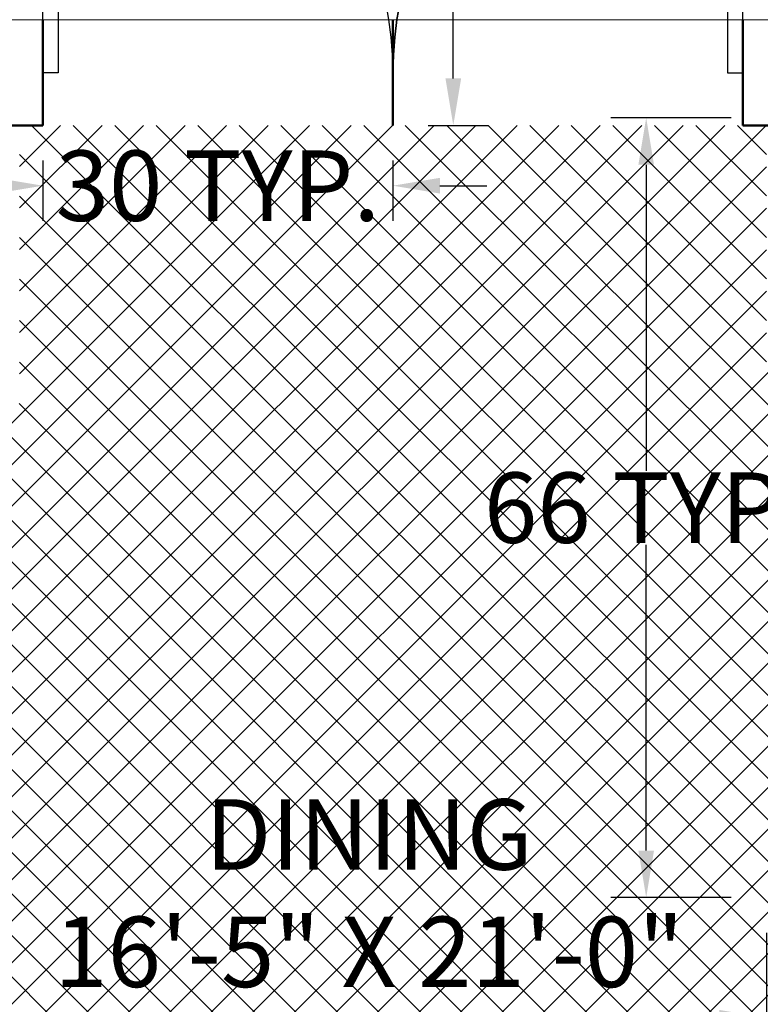
# Model space of a CAD drawing. Units: inches. Extents: x -466983 to 1020, y 324 to 318697.
# Tile 86 of 97: x 679 to 742, y 879 to 963. Entities that reach past the tile are written whole.
import ezdxf

# ---------------------------------------------------------------- set-up
doc = ezdxf.new("R2010")
doc.units = ezdxf.units.IN
doc.header["$MEASUREMENT"] = 0
for name, color, linetype, lineweight in [('A-ANNO-DIMS', 2, 'Continuous', 18), ('A-AREA-IDEN', 7, 'Continuous', 25), ('A-DOOR', 3, 'Continuous', 25), ('A-FLOR-PATT', 252, 'Continuous', 13), ('A-WALL', 7, 'Continuous', 50), ('L-SITE', 3, 'Continuous', 18)]:
    doc.layers.add(name, color=color, linetype=linetype, lineweight=lineweight)
doc.styles.get("Standard").update_dxf_attribs({"font": 'arial.ttf'})
doc.dimstyles.get("Standard").update_dxf_attribs({"dimtxt": 6, "dimasz": 4, "dimexe": 3, "dimexo": 3, "dimgap": 0.09, "dimtad": 0, "dimtih": 1, "dimtoh": 1, "dimdec": 1, "dimzin": 0, "dimdsep": 46, "dimlunit": 3, "dimtxsty": 'Standard', "dimcen": 0.09, "dimadec": 0, "dimazin": 0, "dimtfac": 1, "dimtdec": 1, "dimtofl": 0, "dimtmove": 0, "dimatfit": 3, "dimfxl": 1, "dimtolj": 1, "dimtzin": 0, "dimarcsym": 0})

# ---------------------------------------------------------------- blocks, each defined once
blk = doc.blocks.new('*U39')
for p, q in [((0, 0), (0, -6)), ((-40, 0), (-40, -6))]:
    blk.add_line(p, q)
blk.add_lwpolyline([(0, 0), (0, 40), (-1.75, 40), (-1.75, 0)], close=True)
blk.add_arc((0, 0), 40, 90, 180)
blk = doc.blocks.new('*U41')
for p, q in [((0, 0), (0, -6)), ((40, 0), (40, -6))]:
    blk.add_line(p, q)
blk.add_lwpolyline([(0, 0), (0, 40), (1.75, 40), (1.75, 0)], close=True)
blk.add_arc((0, 0), 40, 0, 90)
blk = doc.blocks.new('DOOR-30IN')
for p, q in [((0, 4.472), (0, 0)), ((29.811, 4.472), (29.811, 0))]:
    blk.add_line(p, q)
blk.add_lwpolyline([(0, 4.472), (0, 34.283), (1.304, 34.283), (1.304, 4.472)], close=True)
blk.add_arc((0, 4.472), 29.812, 0, 90)
blk = doc.blocks.new('*D57')
at = {"layer": 'A-ANNO-DIMS', "color": 0, "lineweight": -2, "transparency": 16777216}
for p, q in [((713.403, 988.221), (718.546, 988.221)), ((715.546, 984.221), (715.546, 974.276)), ((715.546, 957.938), (715.546, 967.883)), ((713.403, 953.938), (718.546, 953.938))]:
    blk.add_line(p, q, dxfattribs=at)
at = {"layer": 'A-ANNO-DIMS', "color": 0, "transparency": 16777216}
for points in [[(714.879, 984.221), (716.213, 984.221), (715.546, 988.221)], [(714.879, 957.938), (716.213, 957.938), (715.546, 953.938)]]:
    blk.add_solid(points, dxfattribs=at)
at = {"layer": 'Defpoints', "color": 0, "transparency": 16777216}
for p in [(710.403, 988.221), (715.546, 988.221), (710.403, 953.938)]:
    blk.add_point(p, dxfattribs=at)
at = {"layer": 'A-ANNO-DIMS', "color": 0, "transparency": 16777216, "insert": (715.546, 971.08), "char_height": 6, "attachment_point": 5}
blk.add_mtext('\\A1;DOOR 34 TYP.', dxfattribs=at)
blk = doc.blocks.new('*D58')
at = {"layer": 'A-ANNO-DIMS', "color": 0, "lineweight": -2, "transparency": 16777216}
for p, q in [((680.592, 950.938), (680.592, 945.795)), ((710.403, 950.938), (710.403, 945.795)), ((676.592, 948.795), (672.592, 948.795)), ((714.403, 948.795), (718.403, 948.795))]:
    blk.add_line(p, q, dxfattribs=at)
at = {"layer": 'A-ANNO-DIMS', "color": 0, "transparency": 16777216}
for points in [[(676.592, 949.462), (676.592, 948.129), (680.592, 948.795)], [(714.403, 949.462), (714.403, 948.129), (710.403, 948.795)]]:
    blk.add_solid(points, dxfattribs=at)
at = {"layer": 'Defpoints', "color": 0, "transparency": 16777216}
for p in [(680.592, 953.938), (710.403, 953.938), (710.403, 948.795)]:
    blk.add_point(p, dxfattribs=at)
at = {"layer": 'A-ANNO-DIMS', "color": 0, "transparency": 16777216, "insert": (695.497, 948.795), "char_height": 6, "attachment_point": 5}
blk.add_mtext('\\A1;30 TYP.', dxfattribs=at)
blk = doc.blocks.new('*D71')
at = {"layer": 'A-ANNO-DIMS', "color": 0, "lineweight": -2, "transparency": 16777216}
for p, q in [((742.215, 885.152), (742.215, 874.91)), ((810.492, 885.152), (810.492, 874.91)), ((738.215, 877.91), (734.215, 877.91)), ((814.492, 877.91), (818.492, 877.91))]:
    blk.add_line(p, q, dxfattribs=at)
at = {"layer": 'A-ANNO-DIMS', "color": 0, "transparency": 16777216}
for points in [[(738.215, 878.577), (738.215, 877.244), (742.215, 877.91)], [(814.492, 878.577), (814.492, 877.244), (810.492, 877.91)]]:
    blk.add_solid(points, dxfattribs=at)
at = {"layer": 'Defpoints', "color": 0, "transparency": 16777216}
for p in [(742.215, 888.152), (810.492, 888.152), (742.215, 877.91)]:
    blk.add_point(p, dxfattribs=at)
at = {"layer": 'A-ANNO-DIMS', "color": 0, "transparency": 16777216, "insert": (776.354, 877.91), "char_height": 6, "attachment_point": 5}
blk.add_mtext('\\A1;L-SOFA 68 TYP.', dxfattribs=at)
blk = doc.blocks.new('*D72')
at = {"layer": 'A-ANNO-DIMS', "color": 0, "lineweight": -2, "transparency": 16777216}
for p, q in [((739.215, 954.575), (728.974, 954.575)), ((731.974, 950.575), (731.974, 924.517)), ((731.974, 892.152), (731.974, 918.21)), ((739.215, 888.152), (728.974, 888.152))]:
    blk.add_line(p, q, dxfattribs=at)
at = {"layer": 'A-ANNO-DIMS', "color": 0, "transparency": 16777216}
for points in [[(731.307, 950.575), (732.641, 950.575), (731.974, 954.575)], [(731.307, 892.152), (732.641, 892.152), (731.974, 888.152)]]:
    blk.add_solid(points, dxfattribs=at)
at = {"layer": 'Defpoints', "color": 0, "transparency": 16777216}
for p in [(731.974, 954.575), (742.215, 954.575), (742.215, 888.152)]:
    blk.add_point(p, dxfattribs=at)
at = {"layer": 'A-ANNO-DIMS', "color": 0, "transparency": 16777216, "insert": (731.974, 921.363), "char_height": 6, "attachment_point": 5}
blk.add_mtext('\\A1;66 TYP.', dxfattribs=at)

msp = doc.modelspace()

# ---------------------------------------------------------------- hatches: boundary and pattern name
at = {"layer": 'A-FLOR-PATT', "transparency": 33554572}
h = msp.add_hatch(dxfattribs=at)
h.set_pattern_fill('ANSI37', color=256, scale=30)
h.set_pattern_definition([(45, (-1212.4137, -290.035), (-2.6516504, 2.6516504), []), (135, (-1212.4137, -290.035), (-2.6516504, -2.6516504), [])])
h.paths.add_polyline_path([(901.806, 1075.938), (900.614, 1075.938), (900.614, 1065.386), (899.391, 1065.386), (898.091, 1065.386), (892.836, 1058.71, -0.258377), (892.188, 1058.351), (879.985, 1058.351, -0.20177), (879.438, 1058.581), (874.081, 1065.386), (872.781, 1065.386), (871.558, 1065.386), (871.558, 1075.938), (813.806, 1075.938), (813.806, 1044.792), (832.395, 1044.792, -0.394795), (848.66, 1028.536), (848.66, 1009.938), (901.806, 1009.938), (901.806, 1015.938), (901.306, 1015.938), (871.306, 1015.938), (871.306, 1017.25), (871.334, 1017.25, -0.401453), (901.306, 1045.938), (901.806, 1045.938)])
edge = h.paths.add_edge_path(flags=16)
edge.add_line((847.773, 1068.949), (847.773, 1073.709))
edge.add_arc((849.227, 1073.709), 1.454, 90, 180, ccw=False)
edge.add_line((849.227, 1075.163), (864.492, 1075.163))
edge.add_arc((864.492, 1073.709), 1.454, 0, 90, ccw=False)
edge.add_line((865.946, 1073.709), (865.946, 1069.004))
edge.add_arc((832.645, 1068.976), 33.301, -20.61234, 0.04725, ccw=False)
edge.add_ellipse((856.859, 1058.48), major_axis=(0, 10.213), ratio=0.685919, start_angle=100.00884, end_angle=259.99116, ccw=False)
edge.add_arc((881.074, 1068.976), 33.301, 180.04725, 200.61234, ccw=False)
h.paths.add_polyline_path([(853.146, 1066.482), (853.146, 1066.453), (853.146, 1066.453, 0.433107), (852.917, 1066.685), (852.917, 1066.453), (853.146, 1066.453), (853.146, 1066.482), (853.088, 1066.612, 0.697939), (852.7, 1066.453), (852.7, 1066.453), (852.7, 1066.482), (852.917, 1067.001), (852.917, 1066.685, -0.396254)], flags=0)
h.paths.add_polyline_path([(861.019, 1066.482), (861.019, 1066.453), (861.019, 1066.453, 0.416404), (860.802, 1066.685), (860.802, 1066.453), (861.019, 1066.453), (861.019, 1066.482), (860.967, 1066.605, 0.713344), (860.573, 1066.453), (860.573, 1066.453), (860.573, 1066.482), (860.802, 1067.001), (860.802, 1066.685, -0.379973)], flags=0)
edge = h.paths.add_edge_path(flags=0)
edge.add_spline(control_points=[(861.13, 1065.785), (861.466, 1065.248), (861.613, 1065.016), (861.983, 1064.374), (862.192, 1063.944), (862.561, 1063.039), (862.721, 1062.563), (862.987, 1061.578), (863.092, 1061.069), (863.245, 1060.031), (863.293, 1059.503), (863.329, 1058.441), (863.318, 1057.908), (863.237, 1056.852), (863.166, 1056.329), (862.97, 1055.308), (862.843, 1054.81), (862.537, 1053.852), (862.357, 1053.393), (861.951, 1052.525), (861.725, 1052.117), (861.233, 1051.362), (860.967, 1051.016), (860.405, 1050.395), (860.108, 1050.12), (859.494, 1049.646), (859.176, 1049.448), (858.528, 1049.13), (858.197, 1049.011), (857.531, 1048.852), (857.196, 1048.812), (856.525, 1048.812), (856.189, 1048.852), (855.524, 1049.01), (855.193, 1049.129), (854.545, 1049.447), (854.227, 1049.645), (853.612, 1050.118), (853.316, 1050.393), (852.753, 1051.014), (852.487, 1051.36), (851.995, 1052.114), (851.769, 1052.523), (851.363, 1053.39), (851.183, 1053.85), (850.877, 1054.807), (850.75, 1055.305), (850.553, 1056.326), (850.483, 1056.849), (850.401, 1057.905), (850.39, 1058.438), (850.426, 1059.5), (850.473, 1060.028), (850.626, 1061.066), (850.732, 1061.575), (850.997, 1062.561), (851.157, 1063.036), (851.525, 1063.942), (851.734, 1064.371), (852.106, 1065.016), (852.254, 1065.25), (852.608, 1065.733)], knot_values=[3.915332, 3.915332, 3.915332, 3.915332, 4.013468, 4.013468, 4.175532, 4.175532, 4.337596, 4.337596, 4.49966, 4.49966, 4.661724, 4.661724, 4.823788, 4.823788, 4.985852, 4.985852, 5.147916, 5.147916, 5.30998, 5.30998, 5.472044, 5.472044, 5.634109, 5.634109, 5.796173, 5.796173, 5.958237, 5.958237, 6.120301, 6.120301, 6.282365, 6.282365, 6.444429, 6.444429, 6.606493, 6.606493, 6.768557, 6.768557, 6.930621, 6.930621, 7.092685, 7.092685, 7.254749, 7.254749, 7.416813, 7.416813, 7.578878, 7.578878, 7.740942, 7.740942, 7.903006, 7.903006, 8.06507, 8.06507, 8.227134, 8.227134, 8.389198, 8.389198, 8.551262, 8.551262, 8.65037, 8.65037, 8.65037, 8.65037], degree=3, periodic=0)
edge.add_line((852.642, 1065.785), (861.13, 1065.785))
edge = h.paths.add_edge_path(flags=0)
edge.add_ellipse((856.85, 1057.743), major_axis=(0, 7.792), ratio=0.687861, start_angle=0, end_angle=360)
h.paths.add_polyline_path([(848.863, 1069.389), (848.863, 1073.96, -0.414214), (849.954, 1075.051), (863.765, 1075.051, -0.414214), (864.856, 1073.96), (864.856, 1069.389, -0.388936), (864.524, 1069.027, -0.043561), (849.195, 1069.027, -0.388936)], flags=0)
h.paths.add_polyline_path([(853.101, 1068.112, -1), (852.677, 1068.112, -1)], flags=0)
edge = h.paths.add_edge_path(flags=0)
edge.add_ellipse((856.859, 1057.338), major_axis=(0, 2.207), ratio=0.657164, start_angle=0, end_angle=360)
h.paths.add_polyline_path([(861.041, 1068.112, -1), (860.618, 1068.112, -1)], flags=0)
edge = h.paths.add_edge_path()
edge.add_line((573.954, 1057.341), (573.954, 1075.938))
edge.add_line((573.954, 1075.938), (558.731, 1075.938))
edge.add_line((558.731, 1075.938), (558.731, 1065.386))
edge.add_line((558.731, 1065.386), (557.507, 1065.386))
edge.add_line((557.507, 1065.386), (556.207, 1065.386))
edge.add_line((556.207, 1065.386), (550.952, 1058.71))
edge.add_arc((550.304, 1059.116), 0.765, 270, 327.94832, ccw=False)
edge.add_line((550.304, 1058.351), (538.101, 1058.351))
edge.add_arc((538.101, 1059.116), 0.765, 224.3704, 270, ccw=False)
edge.add_line((537.555, 1058.581), (532.198, 1065.386))
edge.add_line((532.198, 1065.386), (530.898, 1065.386))
edge.add_line((530.898, 1065.386), (529.674, 1065.386))
edge.add_line((529.674, 1065.386), (529.674, 1075.938))
edge.add_line((529.674, 1075.938), (520.806, 1075.938))
edge.add_line((520.806, 1075.938), (520.806, 1045.938))
edge.add_line((520.806, 1045.938), (521.306, 1045.938))
edge.add_arc((521.306, 1015.938), 30, 2.50749, 90, ccw=False)
edge.add_line((551.277, 1017.25), (551.306, 1017.25))
edge.add_line((551.306, 1017.25), (551.306, 1015.938))
edge.add_line((551.306, 1015.938), (520.806, 1015.938))
edge.add_line((520.806, 1015.938), (520.806, 1009.938))
edge.add_line((520.806, 1009.938), (559.191, 1010.402))
edge.add_arc((559.191, 1011.856), 1.454, 180, 270, ccw=False)
edge.add_line((557.737, 1011.856), (557.737, 1016.561))
edge.add_arc((591.039, 1016.589), 33.301, 159.38766, 180.04725, ccw=False)
edge.add_ellipse((566.824, 1027.085), major_axis=(0, 10.213), ratio=0.685919, start_angle=280.00884, end_angle=439.99116, ccw=False)
edge.add_arc((542.609, 1016.589), 33.301, 0.04725, 20.61234, ccw=False)
edge.add_line((575.91, 1016.616), (575.91, 1011.856))
edge.add_arc((574.456, 1011.856), 1.454, -90, 0, ccw=False)
edge.add_line((574.456, 1010.402), (608.806, 1009.938))
edge.add_line((608.806, 1009.938), (608.806, 1041.086))
edge.add_line((608.806, 1041.086), (590.218, 1041.086))
edge.add_arc((590.775, 1057.907), 16.831, 181.92775, 268.10321, ccw=False)
edge = h.paths.add_edge_path()
edge.add_ellipse((494.244, 583.62), major_axis=(0, 10.213), ratio=0.685919, start_angle=280.00884, end_angle=439.99116, ccw=False)
edge.add_arc((470.03, 573.124), 33.301, 0.04725, 20.61234, ccw=False)
edge.add_line((503.331, 573.152), (503.331, 568.392))
edge.add_arc((501.877, 568.392), 1.454, -90, 0, ccw=False)
edge.add_line((501.877, 566.938), (539.806, 566.938))
edge.add_line((539.806, 566.938), (539.806, 572.938))
edge.add_line((539.806, 572.938), (539.306, 572.938))
edge.add_line((539.306, 572.938), (509.306, 572.938))
edge.add_line((509.306, 572.938), (509.306, 574.25))
edge.add_line((509.306, 574.25), (509.334, 574.25))
edge.add_arc((539.306, 572.938), 30, 90, 177.49251, ccw=False)
edge.add_line((539.306, 602.938), (539.806, 602.938))
edge.add_line((539.806, 602.938), (539.806, 626.938))
edge.add_line((539.806, 626.938), (531.772, 626.938))
edge.add_line((531.772, 626.938), (531.772, 616.386))
edge.add_line((531.772, 616.386), (530.548, 616.386))
edge.add_line((530.548, 616.386), (529.249, 616.386))
edge.add_line((529.249, 616.386), (523.711, 609.351))
edge.add_line((523.711, 609.351), (510.777, 609.351))
edge.add_line((510.777, 609.351), (505.239, 616.386))
edge.add_line((505.239, 616.386), (503.939, 616.386))
edge.add_line((503.939, 616.386), (502.715, 616.386))
edge.add_line((502.715, 616.386), (502.715, 626.938))
edge.add_line((502.715, 626.938), (481.698, 626.938))
edge.add_line((481.698, 626.938), (481.698, 610.995))
edge.add_arc((467.27, 611.473), 14.436, 271.92775, 358.10321, ccw=False)
edge.add_line((467.756, 597.045), (451.806, 597.045))
edge.add_line((451.806, 597.045), (451.806, 584.404))
edge.add_line((451.806, 584.404), (451.806, 566.938))
edge.add_line((451.806, 566.938), (486.612, 566.938))
edge.add_arc((486.612, 568.392), 1.454, 180, 270, ccw=False)
edge.add_line((485.158, 568.392), (485.158, 573.097))
edge.add_arc((518.459, 573.124), 33.301, 159.38766, 180.04725, ccw=False)
h.paths.add_polyline_path([(836.261, 1020.733), (879.89, 1020.733), (879.89, 1039.39), (836.261, 1039.39)], flags=25)
h.paths.add_polyline_path([(549.985, 1036.749), (593.614, 1036.749), (593.614, 1055.407), (549.985, 1055.407)], flags=24)
h.paths.add_polyline_path([(475.123, 595.596), (518.752, 595.596), (518.752, 614.253), (475.123, 614.253)], flags=24)
h = msp.add_hatch(dxfattribs=at)
h.set_pattern_fill('ANSI37', color=256, scale=20)
h.set_pattern_definition([(45, (-1212.4137, -290.035), (-1.767767, 1.767767), []), (135, (-1212.4137, -290.035), (-1.767767, -1.767767), [])])
h.paths.add_polyline_path([(809.806, 870.938), (809.806, 888.152), (806.998, 888.152), (802.662, 888.152), (789.383, 888.152), (786.285, 888.152, -0.414214), (785.499, 888.937), (785.499, 900.196), (785.499, 908.47, -0.414214), (786.808, 909.779, -0.414214), (785.499, 911.088), (785.499, 929.101, -0.414214), (786.808, 930.411, -0.414214), (785.499, 931.72), (785.499, 931.904, -0.414214), (784.19, 930.595), (766.722, 930.595, -0.412359), (765.413, 931.896, -0.413741), (764.115, 930.578), (744.578, 930.422, -0.416556), (743.786, 931.207), (743.786, 933.515), (742.215, 933.515), (742.215, 952.024, -0.001344), (743.786, 952.2), (743.786, 953.938), (678.592, 953.938), (678.592, 951.131), (678.592, 946.794), (678.592, 933.515), (678.592, 930.417, -0.414214), (677.806, 929.631), (666.548, 929.631), (658.274, 929.631, -0.414214), (656.965, 930.94, -0.414214), (655.656, 929.631), (637.642, 929.631, -0.414214), (636.333, 930.94, -0.414214), (635.024, 929.631), (634.839, 929.631, -0.414214), (636.149, 928.322), (636.149, 910.854, -0.412359), (634.848, 909.545, -0.413741), (636.165, 908.247), (636.321, 888.71, -0.416556), (635.536, 887.918), (633.228, 887.918), (633.228, 886.347), (614.719, 886.347, -0.001344), (614.544, 887.918), (612.806, 887.918), (612.806, 834.938), (612.806, 752.938), (612.806, 748.938), (612.806, 697.938), (654.806, 697.938), (654.806, 701.938), (715.806, 701.938), (715.806, 737.435), (774.292, 737.435), (774.292, 795.938), (809.806, 795.938)])
h.paths.add_polyline_path([(679.276, 849.576, 0.102523), (682.148, 849.261, -0.080461), (694.543, 849.773, -0.283899), (694.482, 849.008, 0.136605), (694.407, 848.81, -0.030441), (694.543, 846.893), (694.543, 842.62), (694.543, 838.347, -0.028219), (694.425, 836.568), (694.425, 836.568, 0.196187), (694.446, 836.271, -0.302897), (694.543, 835.467, -0.080461), (682.148, 835.979, 0.102523), (679.276, 835.664, -0.58611), (678.646, 836.017), (678.646, 849.223, -0.58611)], flags=16)
h.paths.add_polyline_path([(679.517, 848.651, 0.699597), (679.476, 848.634, 1.20716), (679.194, 848.742, 0.010621)], flags=0)
h.paths.add_polyline_path([(679.492, 836.561, -0.013798), (679.918, 836.659, -0.071703), (682.853, 837.143, -0.165743), (682.166, 839.101), (682.166, 842.609), (682.166, 846.06, -0.240616), (683.473, 848.677, -0.068263), (693.929, 849.008), (693.788, 848.708), (693.788, 849.023, 0.067332), (683.473, 848.677, 0.240616), (682.166, 846.06), (682.166, 842.609), (682.166, 839.101, 0.23459), (683.461, 836.551, 0.068093), (693.788, 836.195), (693.788, 836.51), (693.93, 836.21, -0.077215), (682.242, 836.782, 0.086627), (679.528, 836.57, -0.628402), (679.503, 836.573), (679.503, 836.607, 0.910458)], flags=0)
h.paths.add_polyline_path([(679.476, 848.636), (679.207, 848.647), (679.207, 836.572, 0.913566), (679.365, 836.586), (679.476, 836.582)], flags=0)
h.paths.add_polyline_path([(679.276, 829.86, 0.102523), (682.148, 829.546, -0.080461), (694.543, 830.057, -0.283899), (694.482, 829.293, 0.136605), (694.407, 829.095, -0.030441), (694.543, 827.178), (694.543, 822.904), (694.543, 818.631, -0.028219), (694.425, 816.853), (694.425, 816.853, 0.196187), (694.446, 816.556, -0.302897), (694.543, 815.752, -0.080461), (682.148, 816.263, 0.102523), (679.276, 815.949, -0.58611), (678.646, 816.302), (678.646, 829.507, -0.58611)], flags=16)
h.paths.add_polyline_path([(679.517, 828.936, 0.699597), (679.476, 828.919, 1.20716), (679.194, 829.027, 0.010621)], flags=0)
h.paths.add_polyline_path([(679.492, 816.846, -0.013798), (679.918, 816.944, -0.071703), (682.853, 817.428, -0.165743), (682.166, 819.385), (682.166, 822.894), (682.166, 826.345, -0.240616), (683.473, 828.961, -0.068263), (693.929, 829.293), (693.788, 828.993), (693.788, 829.308, 0.067332), (683.473, 828.961, 0.240616), (682.166, 826.345), (682.166, 822.894), (682.166, 819.385, 0.23459), (683.461, 816.836, 0.068093), (693.788, 816.48), (693.788, 816.795), (693.93, 816.495, -0.077215), (682.242, 817.066, 0.086627), (679.528, 816.855, -0.628402), (679.503, 816.858), (679.503, 816.892, 0.910458)], flags=0)
h.paths.add_polyline_path([(679.476, 828.921), (679.207, 828.932), (679.207, 816.857, 0.913566), (679.365, 816.871), (679.476, 816.867)], flags=0)
h.paths.add_polyline_path([(679.276, 810.145, 0.102523), (682.148, 809.83, -0.080461), (694.543, 810.342, -0.3023), (694.447, 809.539, 0.10023), (694.406, 809.388, -0.03057), (694.543, 807.462), (694.543, 803.189), (694.543, 798.916, -0.03057), (694.406, 796.991, 0.10023), (694.447, 796.839, -0.3023), (694.543, 796.036, -0.080461), (682.148, 796.548, 0.102523), (679.276, 796.233, -0.58611), (678.646, 796.586), (678.646, 809.792, -0.58611)], flags=16)
h.paths.add_polyline_path([(679.517, 809.242, 0.699597), (679.476, 809.224, 1.20716), (679.194, 809.332, 0.010621)], flags=0)
h.paths.add_polyline_path([(679.492, 797.151, -0.013798), (679.918, 797.25, -0.071703), (682.853, 797.734, -0.165743), (682.166, 799.691), (682.166, 803.2), (682.166, 806.65, -0.239349), (683.461, 809.258, -0.072465), (694.447, 809.541, 0.197932), (694.425, 809.241), (693.788, 809.299), (693.788, 809.614, 0.068093), (683.461, 809.258, 0.239349), (682.166, 806.65), (682.166, 803.2), (682.166, 799.691, 0.235854), (683.473, 797.132, 0.067332), (693.788, 796.786), (693.788, 797.101), (694.425, 797.159, 0.197932), (694.447, 796.859, -0.080419), (682.156, 797.379, 0.083867), (679.528, 797.16, -0.628402), (679.503, 797.164), (679.503, 797.197, 0.910458)], flags=0)
h.paths.add_polyline_path([(679.207, 809.237), (679.207, 797.162, 0.913566), (679.365, 797.176), (679.476, 797.173), (679.476, 809.227)], flags=0)
h.paths.add_polyline_path([(695.364, 853.299), (728.223, 853.299), (728.223, 771.152), (695.364, 771.152)], flags=16)
h.paths.add_polyline_path([(696.021, 852.642), (727.566, 852.642), (727.566, 771.809), (696.021, 771.809)], flags=0)
h.paths.add_polyline_path([(679.276, 788.787, 0.102523), (682.148, 788.472, -0.080461), (694.543, 788.984, -0.3023), (694.447, 788.181, 0.10023), (694.406, 788.03, -0.03057), (694.543, 786.104), (694.543, 781.831), (694.543, 777.558, -0.03057), (694.406, 775.632, 0.10023), (694.447, 775.481, -0.3023), (694.543, 774.678, -0.080461), (682.148, 775.19, 0.102523), (679.276, 774.875, -0.58611), (678.646, 775.228), (678.646, 788.434, -0.58611)], flags=16)
h.paths.add_polyline_path([(679.517, 787.883, 0.699597), (679.476, 787.866, 1.20716), (679.194, 787.974, 0.010621)], flags=0)
h.paths.add_polyline_path([(679.492, 775.793, -0.013798), (679.918, 775.891, -0.071703), (682.853, 776.375, -0.165743), (682.166, 778.333), (682.166, 781.841), (682.166, 785.292, -0.239349), (683.461, 787.899, -0.072465), (694.447, 788.182, 0.197932), (694.425, 787.882), (693.788, 787.94), (693.788, 788.255, 0.068093), (683.461, 787.899, 0.239349), (682.166, 785.292), (682.166, 781.841), (682.166, 778.333, 0.235854), (683.473, 775.774, 0.067332), (693.788, 775.428), (693.788, 775.742), (694.425, 775.8, 0.197932), (694.447, 775.5, -0.080419), (682.156, 776.021, 0.083867), (679.528, 775.802, -0.628402), (679.503, 775.805), (679.503, 775.839, 0.910458)], flags=0)
h.paths.add_polyline_path([(679.207, 787.879), (679.207, 775.804, 0.913566), (679.365, 775.818), (679.476, 775.814), (679.476, 787.868)], flags=0)
h.paths.add_polyline_path([(704.641, 854.12, -0.080461), (705.153, 866.516, 0.102523), (704.838, 869.387, -0.58611), (705.191, 870.017), (718.397, 870.017, -0.58611), (718.75, 869.387, 0.102523), (718.435, 866.516, -0.080461), (718.946, 854.12, -0.3023), (718.144, 854.217, 0.10023), (717.992, 854.257, -0.03057), (716.067, 854.12), (711.794, 854.12), (707.521, 854.12, -0.03057), (705.595, 854.257, 0.10023), (705.444, 854.217, -0.3023)], flags=16)
h.paths.add_polyline_path([(717.846, 869.146, 0.699597), (717.829, 869.187, 1.20716), (717.937, 869.47, 0.010621)], flags=0)
h.paths.add_polyline_path([(705.463, 854.216, -0.080419), (705.984, 866.507, 0.083867), (705.765, 869.135, -0.628402), (705.768, 869.16), (705.802, 869.16, 0.910458), (705.756, 869.171, -0.013798), (705.854, 868.745, -0.071703), (706.338, 865.81, -0.165743), (708.295, 866.497), (711.804, 866.497), (715.255, 866.497, -0.239349), (717.862, 865.202, -0.072465), (718.145, 854.216, 0.197932), (717.845, 854.238), (717.903, 854.876), (718.218, 854.876, 0.068093), (717.862, 865.202, 0.239349), (715.255, 866.497), (711.804, 866.497), (708.295, 866.497, 0.235854), (705.737, 865.19, 0.067332), (705.391, 854.876), (705.705, 854.876), (705.763, 854.238, 0.197932)], flags=16)
h.paths.add_polyline_path([(705.766, 869.456, 0.913566), (705.781, 869.299), (705.777, 869.187), (717.831, 869.187), (717.842, 869.456)], flags=0)
h.paths.add_polyline_path([(729.045, 842.62), (729.045, 846.893, -0.03057), (729.182, 848.818, 0.10023), (729.141, 848.97, -0.3023), (729.045, 849.773, -0.080461), (741.44, 849.261, 0.102523), (744.311, 849.576, -0.58611), (744.942, 849.223), (744.942, 836.017, -0.58611), (744.311, 835.664, 0.102523), (741.44, 835.979, -0.080461), (729.045, 835.467, -0.3023), (729.141, 836.27, 0.10023), (729.182, 836.421, -0.03057), (729.045, 838.347)], flags=16)
h.paths.add_polyline_path([(744.111, 836.585, 1.20716), (744.394, 836.477, 0.010621), (744.07, 836.567, 0.699597)], flags=0)
h.paths.add_polyline_path([(729.141, 836.268, 0.197932), (729.162, 836.568), (729.8, 836.51), (729.8, 836.195, 0.068093), (740.126, 836.551, 0.239349), (741.421, 839.159), (741.421, 842.609), (741.421, 846.118, 0.235854), (740.114, 848.677, 0.067332), (729.8, 849.023), (729.8, 848.708), (729.162, 848.65, 0.197932), (729.141, 848.95, -0.080419), (741.432, 848.43, 0.083867), (744.059, 848.649, -0.628402), (744.085, 848.645), (744.085, 848.612, 0.910458), (744.095, 848.658, -0.013798), (743.67, 848.559, -0.071703), (740.734, 848.075, -0.165743), (741.421, 846.118), (741.421, 842.609), (741.421, 839.159, -0.239349), (740.126, 836.551, -0.072465)], flags=0)
h.paths.add_polyline_path([(729.045, 830.057, -0.080461), (741.44, 829.546, 0.102523), (744.311, 829.86, -0.58611), (744.942, 829.507), (744.942, 816.302, -0.58611), (744.311, 815.949, 0.102523), (741.44, 816.263, -0.080461), (729.045, 815.752, -0.3023), (729.141, 816.554, 0.10023), (729.182, 816.706, -0.03057), (729.045, 818.631), (729.045, 822.904), (729.045, 827.178, -0.03057), (729.182, 829.103, 0.10023), (729.141, 829.255, -0.3023)], flags=16)
h.paths.add_polyline_path([(744.111, 816.869, 1.20716), (744.394, 816.761, 0.010621), (744.07, 816.852, 0.699597)], flags=0)
h.paths.add_polyline_path([(729.141, 829.235, -0.080419), (741.432, 828.714, 0.083867), (744.059, 828.933, -0.628402), (744.085, 828.93), (744.085, 828.896, 0.910458), (744.095, 828.943, -0.013798), (743.67, 828.844, -0.071703), (740.734, 828.36, -0.165743), (741.421, 826.403), (741.421, 822.894), (741.421, 819.443, -0.239349), (740.126, 816.836, -0.072465), (729.141, 816.553, 0.197932), (729.162, 816.853), (729.8, 816.795), (729.8, 816.48, 0.068093), (740.126, 816.836, 0.239349), (741.421, 819.443), (741.421, 822.894), (741.421, 826.403, 0.235854), (740.114, 828.961, 0.067332), (729.8, 829.308), (729.8, 828.993), (729.162, 828.935, 0.197932)], flags=16)
h.paths.add_polyline_path([(729.045, 810.342, -0.080461), (741.44, 809.83, 0.102523), (744.311, 810.145, -0.58611), (744.942, 809.792), (744.942, 796.586, -0.58611), (744.311, 796.233, 0.102523), (741.44, 796.548, -0.080461), (729.045, 796.036, -0.283899), (729.105, 796.801, 0.136605), (729.181, 796.999, -0.030441), (729.045, 798.916), (729.045, 803.189), (729.045, 807.462, -0.028219), (729.163, 809.241), (729.162, 809.241, 0.196187), (729.142, 809.538, -0.302897)], flags=16)
h.paths.add_polyline_path([(744.111, 797.175, 1.20716), (744.394, 797.067, 0.010621), (744.07, 797.158, 0.699597)], flags=0)
h.paths.add_polyline_path([(741.345, 809.027, 0.086627), (744.059, 809.239, -0.628402), (744.085, 809.235), (744.085, 809.202, 0.910458), (744.095, 809.248, -0.013798), (743.67, 809.15, -0.071703), (740.734, 808.666, -0.165743), (741.421, 806.708), (741.421, 803.2), (741.421, 799.749, -0.240616), (740.114, 797.132, -0.068263), (729.658, 796.801), (729.8, 797.101), (729.8, 796.786, 0.067332), (740.114, 797.132, 0.240616), (741.421, 799.749), (741.421, 803.2), (741.421, 806.708, 0.23459), (740.126, 809.258, 0.068093), (729.8, 809.614), (729.8, 809.299), (729.658, 809.599, -0.077215)], flags=0)
h.paths.add_polyline_path([(704.641, 770.33, -0.283899), (705.405, 770.27, 0.136605), (705.603, 770.194, -0.030441), (707.521, 770.33), (711.794, 770.33), (716.067, 770.33, -0.028219), (717.845, 770.212), (717.845, 770.213, 0.196187), (718.143, 770.233, -0.302897), (718.946, 770.33, -0.080461), (718.435, 757.935, 0.102523), (718.75, 755.064, -0.58611), (718.397, 754.433), (705.191, 754.433, -0.58611), (704.838, 755.064, 0.102523), (705.153, 757.935, -0.080461)], flags=16)
h.paths.add_polyline_path([(705.762, 755.305, 0.699597), (705.779, 755.264, 1.20716), (705.671, 754.981, 0.010621)], flags=0)
h.paths.add_polyline_path([(705.405, 769.717), (705.705, 769.575), (705.391, 769.575, 0.067332), (705.737, 759.261, 0.240616), (708.353, 757.954), (711.804, 757.954), (715.313, 757.954, 0.23459), (717.862, 759.249, 0.068093), (718.218, 769.575), (717.903, 769.575), (718.203, 769.717, -0.077215), (717.632, 758.03, 0.086627), (717.843, 755.316, -0.628402), (717.84, 755.29), (717.806, 755.29, 0.910458), (717.853, 755.28, -0.013798), (717.754, 755.705, -0.071703), (717.27, 758.641, -0.165743), (715.313, 757.954), (711.804, 757.954), (708.353, 757.954, -0.240616), (705.737, 759.261, -0.068263)], flags=0)
h.paths.add_polyline_path([(729.045, 788.984, -0.080461), (741.44, 788.472, 0.102523), (744.311, 788.787, -0.58611), (744.942, 788.434), (744.942, 775.228, -0.58611), (744.311, 774.875, 0.102523), (741.44, 775.19, -0.080461), (729.045, 774.678, -0.283899), (729.105, 775.443, 0.136605), (729.181, 775.64, -0.030441), (729.045, 777.558), (729.045, 781.831), (729.045, 786.104, -0.028219), (729.163, 787.882), (729.162, 787.882, 0.196187), (729.142, 788.18, -0.302897)], flags=16)
h.paths.add_polyline_path([(744.111, 775.817, 1.20716), (744.394, 775.709, 0.010621), (744.07, 775.799, 0.699597)], flags=0)
h.paths.add_polyline_path([(741.345, 787.669, 0.086627), (744.059, 787.881, -0.628402), (744.085, 787.877), (744.085, 787.844, 0.910458), (744.095, 787.89, -0.013798), (743.67, 787.791, -0.071703), (740.734, 787.307, -0.165743), (741.421, 785.35), (741.421, 781.841), (741.421, 778.39, -0.240616), (740.114, 775.774, -0.068263), (729.658, 775.443), (729.8, 775.742), (729.8, 775.428, 0.067332), (740.114, 775.774, 0.240616), (741.421, 778.39), (741.421, 781.841), (741.421, 785.35, 0.23459), (740.126, 787.899, 0.068093), (729.8, 788.255), (729.8, 787.94), (729.658, 788.241, -0.077215)], flags=0)
h.paths.add_polyline_path([(744.111, 848.636), (744.111, 836.582), (744.381, 836.572), (744.381, 848.647, 0.913566), (744.223, 848.633)], flags=0)
h.paths.add_polyline_path([(744.223, 828.917), (744.111, 828.921), (744.111, 816.867), (744.381, 816.857), (744.381, 828.932, 0.913566)], flags=0)
h.paths.add_polyline_path([(717.831, 755.264), (705.777, 755.264), (705.766, 754.994), (717.842, 754.994, 0.913566), (717.827, 755.152)], flags=0)
h.paths.add_polyline_path([(744.223, 809.223), (744.111, 809.227), (744.111, 797.173), (744.381, 797.162), (744.381, 809.237, 0.913566)], flags=0)
h.paths.add_polyline_path([(744.111, 787.868), (744.111, 775.814), (744.381, 775.804), (744.381, 787.879, 0.913566), (744.223, 787.865)], flags=0)
h.paths.add_polyline_path([(678.877, 877.123), (737.613, 877.123), (737.613, 899.512), (678.877, 899.512)], flags=24)

# ---------------------------------------------------------------- linework, layer by layer
at = {"layer": 'A-WALL'}
for p, q in [((680.592, 962.938), (680.592, 953.938)), ((710.403, 962.938), (710.403, 953.938)), ((740.215, 962.938), (740.215, 953.938)), ((612.806, 953.938), (680.592, 953.938)), ((740.215, 953.938), (809.806, 953.938))]:
    msp.add_line(p, q, dxfattribs=at)
at = {"layer": 'L-SITE'}
msp.add_line((617.806, 962.938), (804.806, 962.938), dxfattribs=at)

# ---------------------------------------------------------------- block references
at = {"layer": 'A-DOOR'}
for name, p, xscale, yscale, zscale in [('*U41', (680.592, 958.41), 0.7452984294347067, 0.7452984294347067, 0.7452984294347067), ('*U39', (740.215, 958.41), 0.7452984294346952, 0.7452984294346952, 0.7452984294346952)]:
    msp.add_blockref(name, p, dxfattribs=dict(at, xscale=xscale, yscale=yscale, zscale=zscale))
msp.add_blockref('DOOR-30IN', (680.592, 953.938), dxfattribs=at)
msp.add_blockref('DOOR-30IN', (680.592, 953.938), dxfattribs=at)
msp.add_blockref('DOOR-30IN', (680.592, 953.938), dxfattribs=at)
msp.add_blockref('DOOR-30IN', (680.592, 953.938), dxfattribs=at)
at = {"layer": 'A-DOOR', "extrusion": (0, 0, -1), "zscale": -1}
msp.add_blockref('DOOR-30IN', (-740.215, 953.938), dxfattribs=at)
msp.add_blockref('DOOR-30IN', (-740.215, 953.938), dxfattribs=at)

# ---------------------------------------------------------------- texts
at = {"layer": 'A-AREA-IDEN', "insert": (593.589, 896.526), "char_height": 6, "attachment_point": 1}
msp.add_mtext_dynamic_manual_height_columns('\\pxqc;{\\fArial|b1|i0|c0|p34;DINING\\P16\'-5" X 21\'-0"}', width=229.55829, gutter_width=1, heights=[0], dxfattribs=at)

# ---------------------------------------------------------------- dimensions: what is measured, and where the dimension line sits
at = {"layer": 'A-ANNO-DIMS'}
for base, p1, p2, angle, text, picture, middle in [((715.546, 988.221), (710.403, 953.938), (710.403, 988.221), 90, 'DOOR <> TYP.', '*D57', (715.546, 971.08)), ((731.974, 954.575), (742.215, 888.152), (742.215, 954.575), 90, '<> TYP.', '*D72', (731.974, 921.363)), ((742.215, 877.91), (810.492, 888.152), (742.215, 888.152), 180, 'L-SOFA <> TYP.', '*D71', (776.354, 877.91))]:
    dim = msp.add_linear_dim(base=base, p1=p1, p2=p2, angle=angle, text=text, dimstyle='Standard', override={"dimdec": 0, "dimlfac": 1, "dimrnd": 0, "dimzin": 0, "dimdsep": 46, "dimlunit": 2}, dxfattribs=at)
    dim.commit()
    dim.dimension.update_dxf_attribs({"geometry": picture, "text_midpoint": middle})
dim = msp.add_linear_dim(base=(710.403, 948.795), p1=(680.592, 953.938), p2=(710.403, 953.938), text='<> TYP.', dimstyle='Standard', override={"dimdec": 0, "dimlfac": 1, "dimrnd": 0, "dimzin": 0, "dimdsep": 46, "dimlunit": 2}, dxfattribs=at)
dim.commit()
dim.dimension.update_dxf_attribs({"geometry": '*D58', "text_midpoint": (695.497, 948.795)})

doc.saveas('drawing.dxf')
